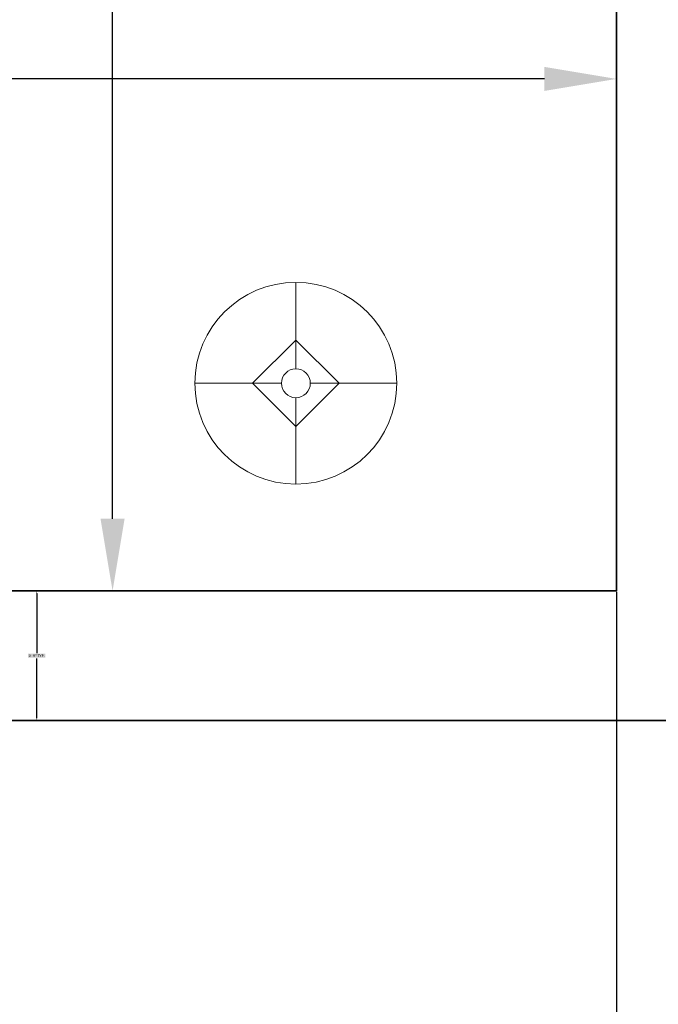
# Model space of a CAD drawing. Units: inches. Extents: x -128 to 854, y -395 to 398.
# Tile 27 of 61: x 263 to 308, y -109 to -41. Entities that reach past the tile are written whole.
import ezdxf

# ---------------------------------------------------------------- set-up
doc = ezdxf.new("R2010")
doc.units = ezdxf.units.IN
doc.header["$MEASUREMENT"] = 0
for name, color, linetype, lineweight in [('A-ANNO-DIMS', 2, 'Continuous', 18), ('A-FURN', 8, 'Continuous', 18), ('A-WALL', 4, 'Continuous', 35)]:
    doc.layers.add(name, color=color, linetype=linetype, lineweight=lineweight)
doc.styles.get("Standard").update_dxf_attribs({"font": 'arial.ttf'})
doc.dimstyles.get("Standard").update_dxf_attribs({"dimtxt": 0.18, "dimasz": 0.18, "dimexe": 0.18, "dimexo": 0.0625, "dimgap": 0.09, "dimtad": 0, "dimtih": 1, "dimtoh": 1, "dimdec": 1, "dimzin": 0, "dimdsep": 46, "dimlunit": 4, "dimtxsty": 'Standard', "dimcen": 0.09, "dimclrd": 1, "dimclre": 2, "dimclrt": 6, "dimadec": 0, "dimazin": 0, "dimtfac": 1, "dimtdec": 1, "dimtofl": 0, "dimtmove": 0, "dimatfit": 3, "dimfxl": 1, "dimtfill": 2, "dimtfillclr": 3, "dimtolj": 1, "dimtzin": 0, "dimarcsym": 0})

# ---------------------------------------------------------------- blocks, each defined once
blk = doc.blocks.new('Lamp - Table')
for p, q in [((0, 7), (0, 1)), ((0, 3), (-3, 0)), ((3, 0), (0, 3)), ((-1, 0), (-7, 0)), ((-3, 0), (0, -3)), ((0, -3), (3, 0)), ((1, 0), (7, 0)), ((0, -1), (0, -7))]:
    blk.add_line(p, q)
for radius in [7, 1]:
    blk.add_circle((0, 0), radius)
blk = doc.blocks.new('*D42')
at = {"layer": 'A-ANNO-DIMS', "color": 0, "lineweight": -2, "transparency": 16777216}
for p, q in [((304.81, 63.741), (269.747, 63.741)), ((269.927, 58.741), (269.927, -6.161)), ((269.927, -75.259), (269.927, -10.358)), ((304.81, -80.259), (269.747, -80.259))]:
    blk.add_line(p, q, dxfattribs=at)
at = {"layer": 'A-ANNO-DIMS', "color": 0, "transparency": 16777216}
for points in [[(269.093, 58.741), (270.76, 58.741), (269.927, 63.741)], [(269.093, -75.259), (270.76, -75.259), (269.927, -80.259)]]:
    blk.add_solid(points, dxfattribs=at)
at = {"layer": 'Defpoints', "color": 0, "transparency": 16777216}
for p in [(269.927, 63.741), (304.873, 63.741), (304.873, -80.259)]:
    blk.add_point(p, dxfattribs=at)
at = {"layer": 'A-ANNO-DIMS', "color": 0, "transparency": 16777216, "insert": (269.927, -8.259), "char_height": 4, "attachment_point": 5, "bg_fill": 1, "box_fill_scale": 1.25, "bg_fill_color": 3, "bg_fill_transparency": 0}
blk.add_mtext("\\A1;12'", dxfattribs=at)
blk = doc.blocks.new('*D43')
at = {"layer": 'A-ANNO-DIMS', "color": 0, "lineweight": -2, "transparency": 16777216}
for p, q in [((156.873, -80.197), (156.873, -44.559)), ((161.873, -44.739), (224.101, -44.739)), ((299.873, -44.739), (237.645, -44.739)), ((304.873, -80.197), (304.873, -44.559))]:
    blk.add_line(p, q, dxfattribs=at)
at = {"layer": 'A-ANNO-DIMS', "color": 0, "transparency": 16777216}
for points in [[(161.873, -43.906), (161.873, -45.572), (156.873, -44.739)], [(299.873, -43.906), (299.873, -45.572), (304.873, -44.739)]]:
    blk.add_solid(points, dxfattribs=at)
at = {"layer": 'Defpoints', "color": 0, "transparency": 16777216}
for p in [(304.873, -44.739), (156.873, -80.259), (304.873, -80.259)]:
    blk.add_point(p, dxfattribs=at)
at = {"layer": 'A-ANNO-DIMS', "color": 0, "transparency": 16777216, "insert": (230.873, -44.739), "char_height": 4, "attachment_point": 5, "bg_fill": 1, "box_fill_scale": 1.25, "bg_fill_color": 3, "bg_fill_transparency": 0}
blk.add_mtext('\\A1;12\'-4"', dxfattribs=at)
blk = doc.blocks.new('*D72')
at = {"layer": 'A-ANNO-DIMS', "color": 2, "lineweight": -2, "transparency": 16777216}
for p, q in [((256.935, -80.259), (264.853, -80.259)), ((256.935, -89.259), (264.853, -89.259))]:
    blk.add_line(p, q, dxfattribs=at)
at = {"layer": 'A-ANNO-DIMS', "color": 1, "lineweight": -2, "transparency": 16777216}
for p, q in [((264.673, -80.439), (264.673, -84.578)), ((264.673, -89.079), (264.673, -84.941))]:
    blk.add_line(p, q, dxfattribs=at)
at = {"layer": 'A-ANNO-DIMS', "color": 1, "transparency": 16777216}
for points in [[(264.643, -80.439), (264.703, -80.439), (264.673, -80.259)], [(264.643, -89.079), (264.703, -89.079), (264.673, -89.259)]]:
    blk.add_solid(points, dxfattribs=at)
at = {"layer": 'Defpoints', "color": 0, "transparency": 16777216}
for p in [(256.873, -80.259), (264.673, -80.259), (256.873, -89.259)]:
    blk.add_point(p, dxfattribs=at)
at = {"layer": 'A-ANNO-DIMS', "color": 6, "transparency": 16777216, "insert": (264.673, -84.759), "char_height": 0.18, "attachment_point": 5, "bg_fill": 1, "box_fill_scale": 1.25, "bg_fill_color": 3, "bg_fill_transparency": 0}
blk.add_mtext('\\A1;0\'-9" TYP.', dxfattribs=at)
blk = doc.blocks.new('*D114')
at = {"layer": 'A-ANNO-DIMS', "color": 2, "lineweight": -2, "transparency": 16777216}
for p, q in [((256.873, -80.322), (256.873, -127.239)), ((304.873, -80.322), (304.873, -127.239))]:
    blk.add_line(p, q, dxfattribs=at)
at = {"layer": 'A-ANNO-DIMS', "color": 1, "lineweight": -2, "transparency": 16777216}
for p, q in [((257.053, -127.059), (280.54, -127.059)), ((304.693, -127.059), (281.206, -127.059))]:
    blk.add_line(p, q, dxfattribs=at)
at = {"layer": 'A-ANNO-DIMS', "color": 1, "transparency": 16777216}
for points in [[(257.053, -127.029), (257.053, -127.089), (256.873, -127.059)], [(304.693, -127.029), (304.693, -127.089), (304.873, -127.059)]]:
    blk.add_solid(points, dxfattribs=at)
at = {"layer": 'Defpoints', "color": 0, "transparency": 16777216}
for p in [(256.873, -80.259), (304.873, -80.259), (256.873, -127.059)]:
    blk.add_point(p, dxfattribs=at)
at = {"layer": 'A-ANNO-DIMS', "color": 6, "transparency": 16777216, "insert": (280.873, -127.059), "char_height": 0.18, "attachment_point": 5, "bg_fill": 1, "box_fill_scale": 1.25, "bg_fill_color": 3, "bg_fill_transparency": 0}
blk.add_mtext('\\A1;4\'-0"', dxfattribs=at)

msp = doc.modelspace()

# ---------------------------------------------------------------- linework, layer by layer
at = {"layer": 'A-WALL'}
for p, q in [((304.873, 63.741), (304.873, -80.259)), ((156.873, -80.259), (304.873, -80.259)), ((156.873, -89.259), (313.873, -89.259))]:
    msp.add_line(p, q, dxfattribs=at)

# ---------------------------------------------------------------- block references
at = {"layer": 'A-FURN'}
msp.add_blockref('Lamp - Table', (282.64, -65.856), dxfattribs=at)

# ---------------------------------------------------------------- dimensions: what is measured, and where the dimension line sits
at = {"layer": 'A-ANNO-DIMS'}
dim = msp.add_linear_dim(base=(269.927, 63.741), p1=(304.873, -80.259), p2=(304.873, 63.741), angle=90, dimstyle='Standard', override={"dimtxt": 4, "dimasz": 5, "dimclrd": 0, "dimclre": 0, "dimclrt": 0}, dxfattribs=at)
dim.commit()
dim.dimension.update_dxf_attribs({"geometry": '*D42', "text_midpoint": (269.927, -8.259)})
for base, p1, p2, override, picture, middle in [((304.873, -44.739), (156.873, -80.259), (304.873, -80.259), {"dimtxt": 4, "dimasz": 5, "dimclrd": 0, "dimclre": 0, "dimclrt": 0}, '*D43', (230.873, -44.739)), ((256.873, -127.059), (304.873, -80.259), (256.873, -80.259), {"dimdec": 1, "dimlfac": 1, "dimrnd": 0, "dimzin": 1, "dimdsep": 46, "dimlunit": 4, "dimfrac": 2}, '*D114', (280.873, -127.059))]:
    dim = msp.add_linear_dim(base=base, p1=p1, p2=p2, dimstyle='Standard', override=override, dxfattribs=at)
    dim.commit()
    dim.dimension.update_dxf_attribs({"geometry": picture, "text_midpoint": middle})
dim = msp.add_linear_dim(base=(264.673, -80.259), p1=(256.873, -89.259), p2=(256.873, -80.259), angle=90, text='<> TYP.', dimstyle='Standard', override={"dimdec": 1, "dimlfac": 1, "dimrnd": 0, "dimzin": 1, "dimdsep": 46, "dimlunit": 4, "dimfrac": 2}, dxfattribs=at)
dim.commit()
dim.dimension.update_dxf_attribs({"geometry": '*D72', "text_midpoint": (264.673, -84.759)})

doc.saveas('drawing.dxf')
